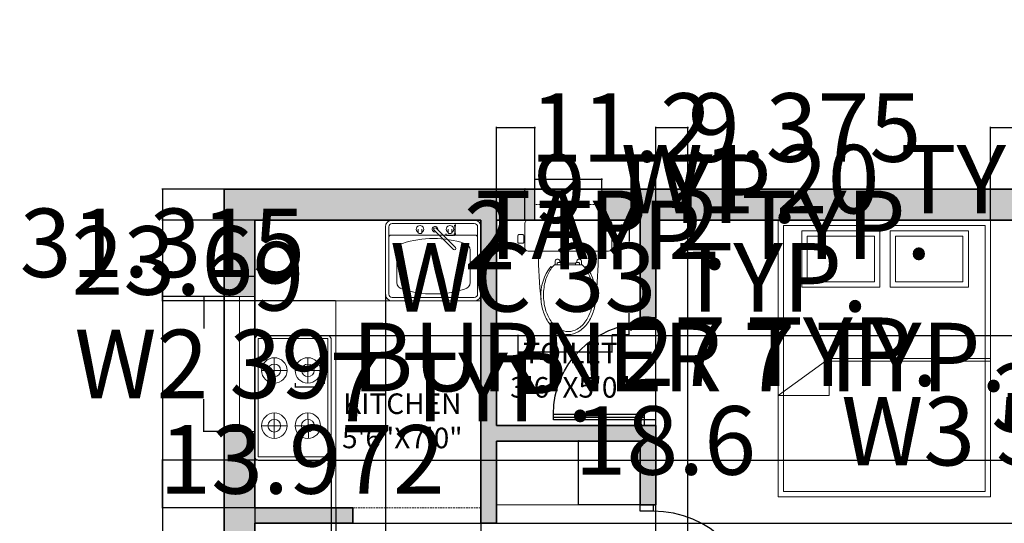
# Model space of a CAD drawing. Units: inches. Extents: x 305 to 776, y 38 to 479.
# Tile 13 of 14: x 331 to 618, y 332 to 479. Entities that reach past the tile are written whole.
import ezdxf

# ---------------------------------------------------------------- set-up
doc = ezdxf.new("R2010")
doc.units = ezdxf.units.IN
doc.header["$MEASUREMENT"] = 0
doc.linetypes.add('DASHED', pattern=[0.75, 0.5, -0.25])
for name, color, linetype, lineweight in [('A-ANNO-DIMS', 2, 'Continuous', 18), ('A-AREA-IDEN', 7, 'Continuous', 18), ('A-DOOR', 4, 'Continuous', 25), ('A-EQPM', 8, 'Continuous', 18), ('A-FLOR-CASE', 8, 'Continuous', 20), ('A-FLOR-FIXT', 9, 'Continuous', 18), ('A-FURN', 8, 'Continuous', 18), ('A-GLAZ', 4, 'Continuous', 20), ('A-GLAZ-OVHD', 4, 'DASHED', 18), ('A-WALL', 7, 'Continuous', 35), ('A-WALL-OVHD', 7, 'DASHED', 18), ('A-WALL-PATT', 252, 'Continuous', 13)]:
    doc.layers.add(name, color=color, linetype=linetype, lineweight=lineweight)
doc.styles.get("Standard").update_dxf_attribs({"font": 'arial.ttf'})
doc.dimstyles.get("Standard").update_dxf_attribs({"dimtxt": 20, "dimasz": 0.18, "dimexe": 0.18, "dimexo": 0.0625, "dimgap": 0.09, "dimtad": 0, "dimtih": 1, "dimtoh": 1, "dimdec": 4, "dimzin": 0, "dimdsep": 46, "dimtxsty": 'Standard', "dimcen": 0.09, "dimadec": 0, "dimazin": 0, "dimtfac": 1, "dimtdec": 4, "dimtofl": 0, "dimtmove": 0, "dimatfit": 3, "dimfxl": 1, "dimtolj": 1, "dimtzin": 0, "dimarcsym": 0})

# ---------------------------------------------------------------- blocks, each defined once
blk = doc.blocks.new('A$C296830DC')
blk.add_line((828.9, 852.6), (828.9, 94.7))
for points in [[(852.6, 94.7), (852.6, 852.6), (805.3, 852.6), (805.3, 94.7)], [(47.4, 94.7), (47.4, 0), (0, 0), (0, 94.7)], [(900, 94.7), (900, 0), (852.6, 0), (852.6, 94.7)]]:
    blk.add_lwpolyline(points, close=True)
blk.add_arc((805.3, 94.7), 757.9, 90, 180)
blk = doc.blocks.new('W1')
blk.add_line((867.01, 338.44), (847.41, 338.44))
blk.add_lwpolyline([(847.41, 333.94), (867.01, 333.94), (867.01, 342.94), (847.41, 342.94)], close=True)
blk = doc.blocks.new('t')
for points in [[(1220.28, 636.63), (1208.55, 636.63, 0.414214), (1207.58, 635.67), (1207.58, 631.86, 0.414214)], [(1220.28, 636.63), (1232.02, 636.63, -0.414214), (1232.98, 635.67), (1232.98, 628.51, -0.414214), (1232.02, 627.55), (1229.53, 627.55)], [(1207.31, 631.86), (1207.31, 632.04, 0.414214), (1206.99, 632.37), (1205.84, 632.37, 0.414214), (1205.52, 632.04), (1205.52, 630.21, 0.414214), (1205.84, 629.89)], [(1205.84, 629.89), (1206.99, 629.89, 0.414214), (1207.31, 630.21), (1207.31, 630.39, 0.414214)], [(1207.31, 630.39), (1207.31, 631.86, 0.414214)], [(1207.58, 631.86), (1207.58, 630.39, 0.414214)], [(1207.58, 630.39), (1207.58, 628.51, 0.414214), (1208.55, 627.55), (1211.03, 627.55)], [(1211.03, 627.55, -0.279901), (1211.54, 626.96, 0.030761), (1212.34, 613.45, 16.522544)], [(1229.53, 627.55, 0.279901), (1229.02, 626.96, -0.030761), (1228.22, 613.45, -16.522544)], [(1216.48, 623.56), (1216.48, 624.75, -0.788198), (1217.76, 624.75), (1217.76, 624.2)], [(1217.03, 623.56), (1217.03, 623.98, -0.414214), (1217.26, 624.2), (1217.94, 624.2, -0.414214), (1218.17, 623.98), (1218.17, 623.56)], [(1223.54, 623.56), (1223.54, 623.98, 0.414214), (1223.31, 624.2), (1222.62, 624.2, 0.414214), (1222.39, 623.98), (1222.39, 623.56)], [(1224.09, 623.56), (1224.09, 624.75, 0.788198), (1222.8, 624.75), (1222.8, 624.2)], [(1212.3, 614.03, -0.186192), (1215.17, 623.1), (1215.53, 622.81)], [(1213.04, 614.76, 0.068564), (1213.62, 610.52, 0.080689), (1215.16, 607.21, 0.107047), (1217.67, 604.81, 0.137952), (1220.28, 604.08, 0.137952), (1222.89, 604.81, 0.107047), (1225.4, 607.21, 0.080689), (1226.94, 610.52, 0.068564), (1227.53, 614.76, 0.068564), (1226.94, 619.01, 0.080689), (1225.4, 622.31, 0.049741), (1224.36, 623.56, 0.137952)], [(1216.2, 623.56, 0.049741), (1215.16, 622.31, 0.080689), (1213.62, 619.01, 0.068564), (1213.04, 614.76, 0.068564)], [(1228.22, 613.45, 0.197511), (1225.39, 623.1), (1225.04, 622.81)], [(1212.27, 614.03, 0.059006), (1212.9, 610.18, 0.081908), (1214.61, 606.59, 0.106902), (1217.38, 604.01, 0.135271), (1220.28, 603.21, 0.135271)], [(1212.34, 613.45, -0.010918), (1212.3, 614.03)], [(1220.28, 603.21, 0.135271), (1223.19, 604.01, 0.106902), (1225.95, 606.59, 0.081908), (1227.66, 610.18, 0.059006), (1228.29, 614.03, 0.070136)]]:
    blk.add_lwpolyline(points, format="xyb")
for points in [[(1207.31, 631.86), (1207.58, 631.86)], [(1207.31, 630.39), (1207.58, 630.39)], [(1211.03, 627.55), (1220.28, 627.55)], [(1229.53, 627.55), (1220.28, 627.55)], [(1218.17, 624.02), (1222.39, 624.02)], [(1216.2, 623.56), (1224.36, 623.56)]]:
    blk.add_lwpolyline(points)
blk = doc.blocks.new('BED')
for p, q in [((1579.44, 254.58), (1564.49, 243.77)), ((1564.49, 243.77), (1579.44, 254.58)), ((1626.49, 254.58), (1579.44, 254.58)), ((1579.44, 254.58), (1579.44, 243.77)), ((1626.49, 253.76), (1579.44, 253.76)), ((1579.44, 243.77), (1564.49, 243.77))]:
    blk.add_line(p, q)
for points in [[(1626.49, 214.2), (1564.49, 214.2), (1564.49, 294.96), (1626.49, 294.96)], [(1624.92, 215.77), (1566.06, 215.77), (1566.06, 293.39), (1624.92, 293.39)], [(1594.24, 275.39), (1571.42, 275.39), (1571.42, 291.78), (1594.24, 291.78)], [(1620.04, 275.39), (1597.22, 275.39), (1597.22, 291.78), (1620.04, 291.78)], [(1592.67, 276.96), (1572.99, 276.96), (1572.99, 290.21), (1592.67, 290.21)], [(1618.47, 276.96), (1598.79, 276.96), (1598.79, 290.21), (1618.47, 290.21)]]:
    blk.add_lwpolyline(points, close=True)
blk = doc.blocks.new('w2')
blk.add_line((795.76, 498.04), (795.76, 458.67))
blk.add_lwpolyline([(791.26, 458.67), (800.26, 458.67), (800.26, 498.04), (791.26, 498.04)], close=True)
blk = doc.blocks.new('COOKTOP-BURNER')
for p, q in [((3.71, 7.42), (3.71, 0)), ((7.42, 3.71), (0, 3.71))]:
    blk.add_line(p, q)
for radius in [3.71, 1.85]:
    blk.add_circle((3.71, 3.71), radius)
blk = doc.blocks.new('FAUCET-HANDLE')
for p, q in [((0.55, 0.18), (0.55, 1.27)), ((1.64, 0.18), (1.64, 1.27))]:
    blk.add_line(p, q)
for centre, radius, start, end in [((1.09, 1.27), 1.09, 300, 240), ((1.09, 0.93), 0.928, 233.9153, 306.0847)]:
    blk.add_arc(centre, radius, start, end)
blk = doc.blocks.new('*D23')
at = {"layer": 'A-ANNO-DIMS', "color": 0, "lineweight": -2, "transparency": 16777216}
for p, q in [((481.33, 429.44), (481.33, 432.5)), ((481.51, 432.32), (500.75, 432.32)), ((500.93, 429.44), (500.93, 432.5)), ((500.93, 432.32), (501.11, 432.32))]:
    blk.add_line(p, q, dxfattribs=at)
at = {"layer": 'A-ANNO-DIMS', "color": 0, "transparency": 16777216}
for points in [[(481.51, 432.35), (481.51, 432.29), (481.33, 432.32)], [(500.75, 432.35), (500.75, 432.29), (500.93, 432.32)]]:
    blk.add_solid(points, dxfattribs=at)
at = {"layer": 'Defpoints', "color": 0, "transparency": 16777216}
for p in [(500.93, 432.32), (481.33, 429.38), (500.93, 429.38)]:
    blk.add_point(p, dxfattribs=at)
at = {"layer": 'A-ANNO-DIMS', "color": 0, "transparency": 16777216, "insert": (575.13, 432.32), "char_height": 20, "attachment_point": 5}
blk.add_mtext('\\A1;W1 20 TYP.', dxfattribs=at)
blk = doc.blocks.new('*D24')
at = {"layer": 'A-ANNO-DIMS', "color": 0, "lineweight": -2, "transparency": 16777216}
for p, q in [((481.27, 429.38), (478.21, 429.38)), ((478.39, 429.38), (478.39, 429.56)), ((478.39, 429.56), (478.57, 429.56)), ((478.39, 420.56), (478.39, 429.2)), ((481.27, 420.38), (478.21, 420.38))]:
    blk.add_line(p, q, dxfattribs=at)
at = {"layer": 'A-ANNO-DIMS', "color": 0, "transparency": 16777216}
for points in [[(478.36, 429.2), (478.42, 429.2), (478.39, 429.38)], [(478.36, 420.56), (478.42, 420.56), (478.39, 420.38)]]:
    blk.add_solid(points, dxfattribs=at)
at = {"layer": 'Defpoints', "color": 0, "transparency": 16777216}
for p in [(478.39, 429.38), (481.33, 429.38), (481.33, 420.38)]:
    blk.add_point(p, dxfattribs=at)
at = {"layer": 'A-ANNO-DIMS', "color": 0, "transparency": 16777216, "insert": (519.57, 429.56), "char_height": 20, "attachment_point": 5}
blk.add_mtext('\\A1;9 TYP.', dxfattribs=at)
blk = doc.blocks.new('*D25')
at = {"layer": 'A-ANNO-DIMS', "color": 0, "lineweight": -2, "transparency": 16777216}
for p, q in [((390.57, 398.07), (384.55, 398.07)), ((384.73, 397.89), (384.73, 388.69)), ((384.73, 358.88), (384.73, 368.07)), ((390.57, 358.7), (384.55, 358.7))]:
    blk.add_line(p, q, dxfattribs=at)
at = {"layer": 'A-ANNO-DIMS', "color": 0, "transparency": 16777216}
for points in [[(384.7, 397.89), (384.76, 397.89), (384.73, 398.07)], [(384.7, 358.88), (384.76, 358.88), (384.73, 358.7)]]:
    blk.add_solid(points, dxfattribs=at)
at = {"layer": 'Defpoints', "color": 0, "transparency": 16777216}
for p in [(384.73, 398.07), (390.63, 398.07), (390.63, 358.7)]:
    blk.add_point(p, dxfattribs=at)
at = {"layer": 'A-ANNO-DIMS', "color": 0, "transparency": 16777216, "insert": (384.73, 378.38), "char_height": 20, "attachment_point": 5}
blk.add_mtext('\\A1;W2 39', dxfattribs=at)
blk = doc.blocks.new('*D26')
at = {"layer": 'A-ANNO-DIMS', "color": 0, "lineweight": -2, "transparency": 16777216}
for p, q in [((390.63, 398.13), (390.63, 404.15)), ((390.81, 403.97), (399.45, 403.97)), ((399.63, 398.13), (399.63, 404.15)), ((399.63, 403.97), (399.81, 403.97))]:
    blk.add_line(p, q, dxfattribs=at)
at = {"layer": 'A-ANNO-DIMS', "color": 0, "transparency": 16777216}
for points in [[(390.81, 404), (390.81, 403.94), (390.63, 403.97)], [(399.45, 404), (399.45, 403.94), (399.63, 403.97)]]:
    blk.add_solid(points, dxfattribs=at)
at = {"layer": 'Defpoints', "color": 0, "transparency": 16777216}
for p in [(399.63, 403.97), (390.63, 398.07), (399.63, 398.07)]:
    blk.add_point(p, dxfattribs=at)
at = {"layer": 'A-ANNO-DIMS', "color": 0, "transparency": 16777216, "insert": (406.48, 403.97), "char_height": 20, "attachment_point": 5}
blk.add_mtext('\\A1;9', dxfattribs=at)
blk = doc.blocks.new('*D27')
at = {"layer": 'A-ANNO-DIMS', "color": 0, "lineweight": -2, "transparency": 16777216}
for p, q in [((630.7, 388.18), (639.63, 388.18)), ((639.45, 388), (639.45, 369.09)), ((639.45, 329.56), (639.45, 348.47)), ((630.7, 329.38), (639.63, 329.38))]:
    blk.add_line(p, q, dxfattribs=at)
at = {"layer": 'A-ANNO-DIMS', "color": 0, "transparency": 16777216}
for points in [[(639.42, 388), (639.48, 388), (639.45, 388.18)], [(639.42, 329.56), (639.48, 329.56), (639.45, 329.38)]]:
    blk.add_solid(points, dxfattribs=at)
at = {"layer": 'Defpoints', "color": 0, "transparency": 16777216}
for p in [(630.63, 388.18), (630.63, 329.38), (639.45, 329.38)]:
    blk.add_point(p, dxfattribs=at)
at = {"layer": 'A-ANNO-DIMS', "color": 0, "transparency": 16777216, "insert": (639.45, 358.78), "char_height": 20, "attachment_point": 5}
blk.add_mtext('\\A1;W3 59 TYP.', dxfattribs=at)
blk = doc.blocks.new('*D31')
at = {"layer": 'A-ANNO-DIMS', "color": 0, "lineweight": -2, "transparency": 16777216}
for p, q in [((503.89, 420.38), (509.03, 420.38)), ((508.85, 420.2), (508.85, 414.11)), ((508.85, 387.14), (508.85, 393.23)), ((503.89, 386.96), (509.03, 386.96))]:
    blk.add_line(p, q, dxfattribs=at)
at = {"layer": 'A-ANNO-DIMS', "color": 0, "transparency": 16777216}
for points in [[(508.82, 420.2), (508.88, 420.2), (508.85, 420.38)], [(508.82, 387.14), (508.88, 387.14), (508.85, 386.96)]]:
    blk.add_solid(points, dxfattribs=at)
at = {"layer": 'Defpoints', "color": 0, "transparency": 16777216}
for p in [(503.83, 420.38), (508.85, 420.38), (503.83, 386.96)]:
    blk.add_point(p, dxfattribs=at)
at = {"layer": 'A-ANNO-DIMS', "color": 0, "transparency": 16777216, "insert": (508.85, 403.67), "char_height": 20, "attachment_point": 5}
blk.add_mtext('\\A1;WC 33 TYP.', dxfattribs=at)
blk = doc.blocks.new('*D32')
at = {"layer": 'A-ANNO-DIMS', "color": 0, "lineweight": -2, "transparency": 16777216}
for p, q in [((476.37, 386.9), (476.37, 381.77)), ((503.83, 386.9), (503.83, 381.77)), ((476.55, 381.95), (503.65, 381.95)), ((503.83, 381.95), (504.01, 381.95))]:
    blk.add_line(p, q, dxfattribs=at)
at = {"layer": 'A-ANNO-DIMS', "color": 0, "transparency": 16777216}
for points in [[(476.55, 381.98), (476.55, 381.92), (476.37, 381.95)], [(503.65, 381.98), (503.65, 381.92), (503.83, 381.95)]]:
    blk.add_solid(points, dxfattribs=at)
at = {"layer": 'Defpoints', "color": 0, "transparency": 16777216}
for p in [(476.37, 386.96), (503.83, 386.96), (503.83, 381.95)]:
    blk.add_point(p, dxfattribs=at)
at = {"layer": 'A-ANNO-DIMS', "color": 0, "transparency": 16777216, "insert": (552.95, 381.95), "char_height": 20, "attachment_point": 5}
blk.add_mtext('\\A1;27 TYP.', dxfattribs=at)
blk = doc.blocks.new('*D41')
at = {"layer": 'A-ANNO-DIMS', "color": 0, "lineweight": -2, "transparency": 16777216}
for p, q in [((418.87, 380.22), (420.1, 380.22)), ((419.92, 380.22), (419.92, 380.4)), ((419.92, 380.4), (420.1, 380.4)), ((419.92, 372.98), (419.92, 380.04)), ((418.87, 372.8), (420.1, 372.8))]:
    blk.add_line(p, q, dxfattribs=at)
at = {"layer": 'A-ANNO-DIMS', "color": 0, "transparency": 16777216}
for points in [[(419.89, 380.04), (419.95, 380.04), (419.92, 380.22)], [(419.89, 372.98), (419.95, 372.98), (419.92, 372.8)]]:
    blk.add_solid(points, dxfattribs=at)
at = {"layer": 'Defpoints', "color": 0, "transparency": 16777216}
for p in [(418.81, 380.22), (419.92, 380.22), (418.81, 372.8)]:
    blk.add_point(p, dxfattribs=at)
at = {"layer": 'A-ANNO-DIMS', "color": 0, "transparency": 16777216, "insert": (523.52, 380.4), "char_height": 20, "attachment_point": 5}
blk.add_mtext('\\A1;BURNER 7 TYP.', dxfattribs=at)
blk = doc.blocks.new('*D42')
at = {"layer": 'A-ANNO-DIMS', "color": 0, "lineweight": -2, "transparency": 16777216}
for p, q in [((411.39, 372.73), (411.39, 371.5)), ((411.57, 371.68), (418.63, 371.68)), ((418.81, 372.73), (418.81, 371.5)), ((418.81, 371.68), (418.99, 371.68))]:
    blk.add_line(p, q, dxfattribs=at)
at = {"layer": 'A-ANNO-DIMS', "color": 0, "transparency": 16777216}
for points in [[(411.57, 371.71), (411.57, 371.65), (411.39, 371.68)], [(418.63, 371.71), (418.63, 371.65), (418.81, 371.68)]]:
    blk.add_solid(points, dxfattribs=at)
at = {"layer": 'Defpoints', "color": 0, "transparency": 16777216}
for p in [(411.39, 372.8), (418.81, 372.8), (418.81, 371.68)]:
    blk.add_point(p, dxfattribs=at)
at = {"layer": 'A-ANNO-DIMS', "color": 0, "transparency": 16777216, "insert": (459.9, 371.68), "char_height": 20, "attachment_point": 5}
blk.add_mtext('\\A1;7 TYP.', dxfattribs=at)
blk = doc.blocks.new('*D43')
at = {"layer": 'A-ANNO-DIMS', "color": 0, "lineweight": -2, "transparency": 16777216}
for p, q in [((457.83, 418.8), (458.31, 418.8)), ((458.13, 418.8), (458.13, 418.98)), ((458.13, 418.98), (458.31, 418.98)), ((458.13, 416.56), (458.13, 418.62)), ((457.83, 416.38), (458.31, 416.38))]:
    blk.add_line(p, q, dxfattribs=at)
at = {"layer": 'A-ANNO-DIMS', "color": 0, "transparency": 16777216}
for points in [[(458.1, 418.62), (458.16, 418.62), (458.13, 418.8)], [(458.1, 416.56), (458.16, 416.56), (458.13, 416.38)]]:
    blk.add_solid(points, dxfattribs=at)
at = {"layer": 'Defpoints', "color": 0, "transparency": 16777216}
for p in [(457.77, 418.8), (458.13, 418.8), (457.77, 416.38)]:
    blk.add_point(p, dxfattribs=at)
at = {"layer": 'A-ANNO-DIMS', "color": 0, "transparency": 16777216, "insert": (530.61, 418.98), "char_height": 20, "attachment_point": 5}
blk.add_mtext('\\A1;TAP 2 TYP.', dxfattribs=at)
blk = doc.blocks.new('*D44')
at = {"layer": 'A-ANNO-DIMS', "color": 0, "lineweight": -2, "transparency": 16777216}
for p, q in [((455.4, 416.31), (455.4, 415.83)), ((455.58, 416.01), (457.59, 416.01)), ((457.77, 416.31), (457.77, 415.83)), ((457.77, 416.01), (457.95, 416.01))]:
    blk.add_line(p, q, dxfattribs=at)
at = {"layer": 'A-ANNO-DIMS', "color": 0, "transparency": 16777216}
for points in [[(455.58, 416.04), (455.58, 415.98), (455.4, 416.01)], [(457.59, 416.04), (457.59, 415.98), (457.77, 416.01)]]:
    blk.add_solid(points, dxfattribs=at)
at = {"layer": 'Defpoints', "color": 0, "transparency": 16777216}
for p in [(455.4, 416.38), (457.77, 416.38), (457.77, 416.01)]:
    blk.add_point(p, dxfattribs=at)
at = {"layer": 'A-ANNO-DIMS', "color": 0, "transparency": 16777216, "insert": (499.12, 416.01), "char_height": 20, "attachment_point": 5}
blk.add_mtext('\\A1;2 TYP.', dxfattribs=at)
blk = doc.blocks.new('*D46')
at = {"layer": 'A-ANNO-DIMS', "color": 0, "lineweight": -2, "transparency": 16777216}
for p, q in [((390.57, 429.38), (372.45, 429.38)), ((372.63, 429.2), (372.63, 259.69)), ((372.63, 69.56), (372.63, 239.07)), ((390.57, 69.38), (372.45, 69.38))]:
    blk.add_line(p, q, dxfattribs=at)
at = {"layer": 'A-ANNO-DIMS', "color": 0, "transparency": 16777216}
for points in [[(372.6, 429.2), (372.66, 429.2), (372.63, 429.38)], [(372.6, 69.56), (372.66, 69.56), (372.63, 69.38)]]:
    blk.add_solid(points, dxfattribs=at)
at = {"layer": 'Defpoints', "color": 0, "transparency": 16777216}
for p in [(372.63, 429.38), (390.63, 429.38), (390.63, 69.38)]:
    blk.add_point(p, dxfattribs=at)
at = {"layer": 'A-ANNO-DIMS', "color": 0, "transparency": 16777216, "insert": (372.63, 249.38), "char_height": 20, "attachment_point": 5}
blk.add_mtext('\\A1;360', dxfattribs=at)
blk = doc.blocks.new('*D49')
at = {"layer": 'A-ANNO-DIMS', "color": 0, "lineweight": -2, "transparency": 16777216}
for p, q in [((399.7, 331.88), (648.81, 331.88)), ((648.63, 331.7), (648.63, 330.88)), ((399.7, 309.28), (648.81, 309.28)), ((648.63, 309.46), (648.63, 310.28))]:
    blk.add_line(p, q, dxfattribs=at)
at = {"layer": 'A-ANNO-DIMS', "color": 0, "transparency": 16777216}
for points in [[(648.6, 331.7), (648.66, 331.7), (648.63, 331.88)], [(648.6, 309.46), (648.66, 309.46), (648.63, 309.28)]]:
    blk.add_solid(points, dxfattribs=at)
at = {"layer": 'Defpoints', "color": 0, "transparency": 16777216}
for p in [(399.63, 331.88), (648.63, 331.88), (399.63, 309.28)]:
    blk.add_point(p, dxfattribs=at)
at = {"layer": 'A-ANNO-DIMS', "color": 0, "transparency": 16777216, "insert": (648.63, 320.58), "char_height": 20, "attachment_point": 5}
blk.add_mtext('\\A1;22.6', dxfattribs=at)
blk = doc.blocks.new('*D50')
at = {"layer": 'A-ANNO-DIMS', "color": 0, "lineweight": -2, "transparency": 16777216}
for p, q in [((390.57, 429.38), (372.45, 429.38)), ((372.63, 429.2), (372.63, 424.03)), ((372.63, 398.25), (372.63, 403.42)), ((390.57, 398.07), (372.45, 398.07))]:
    blk.add_line(p, q, dxfattribs=at)
at = {"layer": 'A-ANNO-DIMS', "color": 0, "transparency": 16777216}
for points in [[(372.6, 429.2), (372.66, 429.2), (372.63, 429.38)], [(372.6, 398.25), (372.66, 398.25), (372.63, 398.07)]]:
    blk.add_solid(points, dxfattribs=at)
at = {"layer": 'Defpoints', "color": 0, "transparency": 16777216}
for p in [(390.63, 429.38), (372.63, 398.07), (390.63, 398.07)]:
    blk.add_point(p, dxfattribs=at)
at = {"layer": 'A-ANNO-DIMS', "color": 0, "transparency": 16777216, "insert": (372.63, 413.72), "char_height": 20, "attachment_point": 5}
blk.add_mtext('\\A1;31.315', dxfattribs=at)
blk = doc.blocks.new('*D54')
at = {"layer": 'A-ANNO-DIMS', "color": 0, "lineweight": -2, "transparency": 16777216}
for p, q in [((470.13, 420.44), (470.13, 447.56)), ((470.31, 447.38), (481.15, 447.38)), ((481.33, 420.44), (481.33, 447.56)), ((481.33, 447.38), (481.51, 447.38))]:
    blk.add_line(p, q, dxfattribs=at)
at = {"layer": 'A-ANNO-DIMS', "color": 0, "transparency": 16777216}
for points in [[(470.31, 447.41), (470.31, 447.35), (470.13, 447.38)], [(481.15, 447.41), (481.15, 447.35), (481.33, 447.38)]]:
    blk.add_solid(points, dxfattribs=at)
at = {"layer": 'Defpoints', "color": 0, "transparency": 16777216}
for p in [(481.33, 447.38), (470.13, 420.38), (481.33, 420.38)]:
    blk.add_point(p, dxfattribs=at)
at = {"layer": 'A-ANNO-DIMS', "color": 0, "transparency": 16777216, "insert": (506.53, 447.38), "char_height": 20, "attachment_point": 5}
blk.add_mtext('\\A1;11.2', dxfattribs=at)
blk = doc.blocks.new('*D58')
at = {"layer": 'A-ANNO-DIMS', "color": 0, "lineweight": -2, "transparency": 16777216}
for p, q in [((516.63, 138.44), (516.63, 447.56)), ((516.81, 447.38), (525.83, 447.38)), ((526.01, 138.44), (526.01, 447.56)), ((526.01, 447.38), (526.19, 447.38))]:
    blk.add_line(p, q, dxfattribs=at)
at = {"layer": 'A-ANNO-DIMS', "color": 0, "transparency": 16777216}
for points in [[(516.81, 447.41), (516.81, 447.35), (516.63, 447.38)], [(525.83, 447.41), (525.83, 447.35), (526.01, 447.38)]]:
    blk.add_solid(points, dxfattribs=at)
at = {"layer": 'Defpoints', "color": 0, "transparency": 16777216}
for p in [(526.01, 447.38), (516.63, 138.38), (526.01, 138.38)]:
    blk.add_point(p, dxfattribs=at)
at = {"layer": 'A-ANNO-DIMS', "color": 0, "transparency": 16777216, "insert": (560.1, 447.38), "char_height": 20, "attachment_point": 5}
blk.add_mtext('\\A1;9.375', dxfattribs=at)
blk = doc.blocks.new('*D61')
at = {"layer": 'A-ANNO-DIMS', "color": 0, "lineweight": -2, "transparency": 16777216}
for p, q in [((437.73, 398.69), (437.73, 51.2)), ((465.63, 398.69), (465.63, 51.2)), ((437.91, 51.38), (465.45, 51.38)), ((465.63, 51.38), (465.81, 51.38))]:
    blk.add_line(p, q, dxfattribs=at)
at = {"layer": 'A-ANNO-DIMS', "color": 0, "transparency": 16777216}
for points in [[(437.91, 51.41), (437.91, 51.35), (437.73, 51.38)], [(465.45, 51.41), (465.45, 51.35), (465.63, 51.38)]]:
    blk.add_solid(points, dxfattribs=at)
at = {"layer": 'Defpoints', "color": 0, "transparency": 16777216}
for p in [(437.73, 398.75), (465.63, 398.75), (465.63, 51.38)]:
    blk.add_point(p, dxfattribs=at)
at = {"layer": 'A-ANNO-DIMS', "color": 0, "transparency": 16777216, "insert": (492.07, 51.38), "char_height": 20, "attachment_point": 5}
blk.add_mtext('\\A1;27.9', dxfattribs=at)
blk = doc.blocks.new('*D62')
at = {"layer": 'A-ANNO-DIMS', "color": 0, "lineweight": -2, "transparency": 16777216}
for p, q in [((399.63, 336.32), (399.63, 51.2)), ((423.23, 336.32), (423.23, 51.2)), ((399.81, 51.38), (423.05, 51.38)), ((423.23, 51.38), (423.41, 51.38))]:
    blk.add_line(p, q, dxfattribs=at)
at = {"layer": 'A-ANNO-DIMS', "color": 0, "transparency": 16777216}
for points in [[(399.81, 51.41), (399.81, 51.35), (399.63, 51.38)], [(423.05, 51.41), (423.05, 51.35), (423.23, 51.38)]]:
    blk.add_solid(points, dxfattribs=at)
at = {"layer": 'Defpoints', "color": 0, "transparency": 16777216}
for p in [(399.63, 336.38), (423.23, 336.38), (423.23, 51.38)]:
    blk.add_point(p, dxfattribs=at)
at = {"layer": 'A-ANNO-DIMS', "color": 0, "transparency": 16777216, "insert": (449.64, 51.38), "char_height": 20, "attachment_point": 5}
blk.add_mtext('\\A1;23.6', dxfattribs=at)
blk = doc.blocks.new('*D63')
at = {"layer": 'A-ANNO-DIMS', "color": 0, "lineweight": -2, "transparency": 16777216}
for p, q in [((399.57, 420.38), (372.45, 420.38)), ((372.63, 420.2), (372.63, 418.89)), ((423.17, 396.78), (372.45, 396.78)), ((372.63, 396.96), (372.63, 398.27))]:
    blk.add_line(p, q, dxfattribs=at)
at = {"layer": 'A-ANNO-DIMS', "color": 0, "transparency": 16777216}
for points in [[(372.6, 420.2), (372.66, 420.2), (372.63, 420.38)], [(372.6, 396.96), (372.66, 396.96), (372.63, 396.78)]]:
    blk.add_solid(points, dxfattribs=at)
at = {"layer": 'Defpoints', "color": 0, "transparency": 16777216}
for p in [(372.63, 420.38), (399.63, 420.38), (423.23, 396.78)]:
    blk.add_point(p, dxfattribs=at)
at = {"layer": 'A-ANNO-DIMS', "color": 0, "transparency": 16777216, "insert": (372.63, 408.58), "char_height": 20, "attachment_point": 5}
blk.add_mtext('\\A1;23.6', dxfattribs=at)
blk = doc.blocks.new('*D64')
at = {"layer": 'A-ANNO-DIMS', "color": 0, "lineweight": -2, "transparency": 16777216}
for p, q in [((400.62, 386.71), (648.81, 386.71)), ((648.63, 386.53), (648.63, 378.84)), ((648.63, 350.53), (648.63, 358.22)), ((400.62, 350.35), (648.81, 350.35))]:
    blk.add_line(p, q, dxfattribs=at)
at = {"layer": 'A-ANNO-DIMS', "color": 0, "transparency": 16777216}
for points in [[(648.6, 386.53), (648.66, 386.53), (648.63, 386.71)], [(648.6, 350.53), (648.66, 350.53), (648.63, 350.35)]]:
    blk.add_solid(points, dxfattribs=at)
at = {"layer": 'Defpoints', "color": 0, "transparency": 16777216}
for p in [(400.56, 386.71), (648.63, 386.71), (400.56, 350.35)]:
    blk.add_point(p, dxfattribs=at)
at = {"layer": 'A-ANNO-DIMS', "color": 0, "transparency": 16777216, "insert": (648.63, 368.53), "char_height": 20, "attachment_point": 5}
blk.add_mtext('\\A1;36.35', dxfattribs=at)
blk = doc.blocks.new('*D65')
at = {"layer": 'A-ANNO-DIMS', "color": 0, "lineweight": -2, "transparency": 16777216}
for p, q in [((399.63, 351.22), (399.63, 51.2)), ((421.89, 351.22), (421.89, 51.2)), ((399.81, 51.38), (421.71, 51.38)), ((421.89, 51.38), (422.07, 51.38))]:
    blk.add_line(p, q, dxfattribs=at)
at = {"layer": 'A-ANNO-DIMS', "color": 0, "transparency": 16777216}
for points in [[(399.81, 51.41), (399.81, 51.35), (399.63, 51.38)], [(421.71, 51.41), (421.71, 51.35), (421.89, 51.38)]]:
    blk.add_solid(points, dxfattribs=at)
at = {"layer": 'Defpoints', "color": 0, "transparency": 16777216}
for p in [(399.63, 351.28), (421.89, 351.28), (421.89, 51.38)]:
    blk.add_point(p, dxfattribs=at)
at = {"layer": 'A-ANNO-DIMS', "color": 0, "transparency": 16777216, "insert": (463.84, 51.38), "char_height": 20, "attachment_point": 5}
blk.add_mtext('\\A1;22.257', dxfattribs=at)
blk = doc.blocks.new('*D66')
at = {"layer": 'A-ANNO-DIMS', "color": 0, "lineweight": -2, "transparency": 16777216}
for p, q in [((400.5, 350.35), (372.45, 350.35)), ((372.63, 350.35), (372.63, 350.53)), ((372.63, 350.53), (372.81, 350.53)), ((372.63, 336.56), (372.63, 350.17)), ((423.17, 336.38), (372.45, 336.38))]:
    blk.add_line(p, q, dxfattribs=at)
at = {"layer": 'A-ANNO-DIMS', "color": 0, "transparency": 16777216}
for points in [[(372.6, 350.17), (372.66, 350.17), (372.63, 350.35)], [(372.6, 336.56), (372.66, 336.56), (372.63, 336.38)]]:
    blk.add_solid(points, dxfattribs=at)
at = {"layer": 'Defpoints', "color": 0, "transparency": 16777216}
for p in [(372.63, 350.35), (400.56, 350.35), (423.23, 336.38)]:
    blk.add_point(p, dxfattribs=at)
at = {"layer": 'A-ANNO-DIMS', "color": 0, "transparency": 16777216, "insert": (413.37, 350.53), "char_height": 20, "attachment_point": 5}
blk.add_mtext('\\A1;13.972', dxfattribs=at)
blk = doc.blocks.new('*D68')
at = {"layer": 'A-ANNO-DIMS', "color": 0, "lineweight": -2, "transparency": 16777216}
for p, q in [((614.36, 420.44), (614.36, 447.56)), ((614.54, 447.38), (621.45, 447.38)), ((621.63, 420.44), (621.63, 447.56)), ((621.63, 447.38), (621.81, 447.38))]:
    blk.add_line(p, q, dxfattribs=at)
at = {"layer": 'A-ANNO-DIMS', "color": 0, "transparency": 16777216}
for points in [[(614.54, 447.41), (614.54, 447.35), (614.36, 447.38)], [(621.45, 447.41), (621.45, 447.35), (621.63, 447.38)]]:
    blk.add_solid(points, dxfattribs=at)
at = {"layer": 'Defpoints', "color": 0, "transparency": 16777216}
for p in [(621.63, 447.38), (614.36, 420.38), (621.63, 420.38)]:
    blk.add_point(p, dxfattribs=at)
at = {"layer": 'A-ANNO-DIMS', "color": 0, "transparency": 16777216, "insert": (653.64, 447.38), "char_height": 20, "attachment_point": 5}
blk.add_mtext('\\A1;7.271', dxfattribs=at)
blk = doc.blocks.new('*D71')
at = {"layer": 'A-ANNO-DIMS', "color": 0, "lineweight": -2, "transparency": 16777216}
for p, q in [((512.07, 355.88), (493.95, 355.88)), ((494.13, 355.88), (494.13, 356.06)), ((494.13, 356.06), (494.31, 356.06)), ((494.13, 337.46), (494.13, 355.7)), ((512.07, 337.28), (493.95, 337.28))]:
    blk.add_line(p, q, dxfattribs=at)
at = {"layer": 'A-ANNO-DIMS', "color": 0, "transparency": 16777216}
for points in [[(494.1, 355.7), (494.16, 355.7), (494.13, 355.88)], [(494.1, 337.46), (494.16, 337.46), (494.13, 337.28)]]:
    blk.add_solid(points, dxfattribs=at)
at = {"layer": 'Defpoints', "color": 0, "transparency": 16777216}
for p in [(494.13, 355.88), (512.13, 355.88), (512.13, 337.28)]:
    blk.add_point(p, dxfattribs=at)
at = {"layer": 'A-ANNO-DIMS', "color": 0, "transparency": 16777216, "insert": (519.43, 356.06), "char_height": 20, "attachment_point": 5}
blk.add_mtext('\\A1;18.6', dxfattribs=at)

msp = doc.modelspace()

# ---------------------------------------------------------------- hatches: boundary and pattern name
at = {"layer": 'A-WALL-PATT'}
h = msp.add_hatch(color=256, dxfattribs=at)
h.dxf.hatch_style = 1
h.paths.add_polyline_path([(481.3329, 429.382), (390.6329, 429.382), (390.6329, 398.067), (399.6329, 398.067), (399.6329, 420.382), (465.6329, 420.382), (465.6329, 331.882), (470.1329, 331.882), (470.1329, 355.882), (512.1329, 355.882), (512.1329, 337.282), (512.1329, 337.282), (515.8592, 337.282), (516.6329, 337.282), (516.6329, 360.382), (513.3171, 360.382), (470.1329, 360.382), (470.1329, 420.382), (481.3329, 420.382)])
h.paths.add_polyline_path([(630.6329, 429.382), (500.9329, 429.382), (500.9329, 420.382), (502.8693, 420.382), (512.1329, 420.382), (512.1329, 391.882), (516.6329, 391.882), (516.6329, 420.382), (621.6329, 420.382), (621.6329, 388.182), (630.6329, 388.182)])
h.paths.add_polyline_path([(630.6329, 329.382), (621.6329, 329.382), (621.6329, 301.882), (512.1329, 301.882), (512.1329, 297.382), (515.8592, 297.382), (557.6329, 297.382), (621.6329, 297.382), (621.6329, 286.182), (630.6329, 286.182)])
h.paths.add_polyline_path([(630.6329, 266.582), (621.6329, 266.582), (621.6329, 255.382), (589.1329, 255.382), (589.1329, 250.882), (621.6329, 250.882), (621.6329, 226.282), (630.6329, 226.282)])
h.paths.add_polyline_path([(630.6329, 167.482), (621.6329, 167.482), (621.6329, 149.1444), (621.6329, 142.882), (516.6329, 142.882), (516.6329, 261.982), (512.1329, 261.982), (512.1329, 138.382), (621.6329, 138.382), (621.6329, 78.382), (512.1329, 78.382), (512.1329, 69.382), (630.6329, 69.382)])
h.paths.add_polyline_path([(464.1329, 138.382), (476.7329, 138.382), (476.7329, 142.1084), (476.7329, 142.882), (459.6329, 142.882), (459.6329, 78.382), (399.6329, 78.382), (399.6329, 98.582), (390.6329, 98.582), (390.6329, 69.382), (464.1329, 69.382)])
h.paths.add_polyline_path([(459.6329, 142.882), (439.3329, 142.882), (439.3329, 138.382), (459.6329, 138.382)], flags=17)
h.paths.add_polyline_path([(399.6329, 138.382), (403.9329, 138.382), (403.9329, 141.5545), (403.9329, 141.5545), (403.9329, 142.882), (399.6329, 142.882), (399.6329, 250.4819), (390.6329, 250.4819), (390.6329, 118.182), (399.6329, 118.182)])
h.paths.add_polyline_path([(399.6329, 331.882), (428.2629, 331.882), (428.2629, 336.382), (399.6329, 336.382), (399.6329, 358.697), (390.6329, 358.697), (390.6329, 309.2819), (399.6329, 309.2819)])

# ---------------------------------------------------------------- linework, layer by layer
at = {"layer": 'A-EQPM'}
for p, q in [((399.6329, 386.7066), (399.6329, 350.3541)), ((400.5603, 386.7066), (420.9622, 386.7066)), ((400.5603, 385.7793), (400.5603, 351.2815)), ((400.5603, 385.7793), (420.9622, 385.7793)), ((420.9622, 386.7066), (420.9622, 386.7016)), ((420.9622, 385.7793), (420.9622, 351.2815)), ((421.8895, 385.7834), (421.8895, 351.2815)), ((415.0965, 364.0791), (415.2527, 356.6635)), ((405.3095, 360.3696), (409.0189, 360.3696)), ((418.806, 360.3696), (411.3871, 360.3696)), ((400.5603, 351.2815), (420.9622, 351.2815)), ((400.3441, 350.3541), (420.9622, 350.3541))]:
    msp.add_line(p, q, dxfattribs=at)
for radius in [3.7094, 1.8547]:
    msp.add_circle((415.0965, 360.3696), radius, dxfattribs=at)
for centre, radius, start, end in [((400.9641, 385.3755), 1.391, 106.874566, 163.125441), ((420.4738, 385.2809), 1.5022, 19.539718, 72.137641), ((400.4522, 351.1734), 0.8264, 172.484866, 277.515134), ((420.5584, 351.6853), 1.391, 286.874555, 343.125445)]:
    msp.add_arc(centre, radius, start, end, dxfattribs=at)
at = {"layer": 'A-FLOR-CASE'}
for p, q in [((465.6329, 396.782), (423.2329, 396.782)), ((423.2329, 396.782), (423.2329, 336.382)), ((512.1329, 337.282), (470.1329, 337.282))]:
    msp.add_line(p, q, dxfattribs=at)
at = {"layer": 'A-FLOR-FIXT'}
for p, q in [((463.6662, 420.382), (439.697, 420.382)), ((437.7303, 418.4154), (437.7303, 398.7487)), ((439.697, 419.3987), (463.6662, 419.3987)), ((451.9261, 417.4155), (457.5756, 411.766)), ((458.155, 412.3454), (452.5056, 417.9949)), ((465.6329, 398.7487), (465.6329, 418.4154)), ((463.9297, 416.0117), (439.3692, 416.0117)), ((441.6343, 416.0117), (439.3692, 416.0117)), ((441.0665, 411.5867), (441.0665, 402.1904)), ((462.4813, 402.1904), (462.4813, 411.5867)), ((439.697, 397.7654), (463.6662, 397.7654)), ((463.6662, 396.782), (439.697, 396.782))]:
    msp.add_line(p, q, dxfattribs=at)
for points in [[(438.7136, 418.4154), (438.7136, 398.7487)], [(464.6496, 398.7487), (464.6496, 418.4154)]]:
    msp.add_lwpolyline(points, dxfattribs=at)
for points in [[(442.7276, 413.5748, -0.15464107), (460.8202, 413.5748)], [(442.7276, 400.2023, 0.15464107), (460.8202, 400.2023, -0.02214818)]]:
    msp.add_lwpolyline(points, format="xyb", dxfattribs=at)
for centre, radius, start, end in [((439.697, 418.4154), 1.9667, 90, 180), ((463.6662, 418.4154), 1.9667, 0, 90), ((439.697, 418.4154), 0.9833, 90, 180), ((452.2158, 417.7052), 0.8194, 345, 285), ((452.2158, 417.7052), 0.4097, 45, 225), ((463.6662, 418.4154), 0.9833, 0, 90), ((439.3692, 415.3561), 0.6556, 90, 180), ((463.994, 415.3561), 0.6556, 0, 90), ((443.1051, 411.5713), 2.0387, 100.670755, 179.56936), ((457.8653, 412.0557), 0.4097, 225, 45), ((460.4427, 411.5713), 2.0387, 0.43064, 79.329245), ((443.1051, 402.2057), 2.0387, 180.43064, 259.329245), ((460.4427, 402.2057), 2.0387, 280.670755, 359.56936), ((439.697, 398.7487), 1.9667, 180, 270), ((439.697, 398.7487), 0.9833, 180, 270), ((463.6662, 398.7487), 1.9667, 270, 0), ((463.6662, 398.7487), 0.9833, 270, 0)]:
    msp.add_arc(centre, radius, start, end, dxfattribs=at)
at = {"layer": 'A-WALL'}
for p, q in [((399.6329, 420.382), (399.6329, 336.382)), ((465.6329, 420.382), (399.6329, 420.382)), ((465.6329, 420.382), (465.6329, 331.882)), ((470.1329, 420.382), (470.1329, 360.382)), ((512.1329, 420.382), (470.1329, 420.382)), ((512.1329, 420.382), (512.1329, 391.882)), ((621.6329, 420.382), (516.6329, 420.382)), ((516.6329, 420.382), (516.6329, 391.882)), ((516.6329, 391.882), (512.1329, 391.882)), ((516.6329, 360.382), (470.1329, 360.382)), ((516.6329, 360.382), (516.6329, 337.282)), ((512.1329, 355.882), (470.1329, 355.882)), ((470.1329, 355.882), (470.1329, 331.882)), ((512.1329, 355.882), (512.1329, 337.282)), ((428.2629, 336.382), (399.6329, 336.382)), ((428.2629, 336.382), (428.2629, 331.882)), ((516.6329, 337.282), (512.1329, 337.282)), ((399.6329, 331.882), (399.6329, 142.882)), ((428.2629, 331.882), (399.6329, 331.882)), ((470.1329, 331.882), (465.6329, 331.882))]:
    msp.add_line(p, q, dxfattribs=at)
msp.add_lwpolyline([(390.6329, 69.382), (630.6329, 69.382), (630.6329, 429.382), (390.6329, 429.382)], close=True, dxfattribs=at)
at = {"layer": 'A-WALL-OVHD'}
for p, q in [((428.2629, 336.382), (465.6329, 336.382)), ((465.6329, 331.882), (428.2629, 331.882))]:
    msp.add_line(p, q, dxfattribs=at)

# ---------------------------------------------------------------- block references
at = {"layer": 'A-DOOR'}
for p, xscale, yscale, zscale, rotation in [((516.6329, 391.882), -0.035, 0.035, 0.035, 90), ((512.1329, 337.282), 0.0393333333333333, 0.0393333333333333, 0.0393333333333333, 270)]:
    msp.add_blockref('A$C296830DC', p, dxfattribs=dict(at, xscale=xscale, yscale=yscale, zscale=zscale, rotation=rotation))
at = {"layer": 'A-EQPM'}
for p, rotation in [((409.0189, 372.7962), 90.00000000000088), ((401.6, 364.0791), 270.0000000000009)]:
    msp.add_blockref('COOKTOP-BURNER', p, dxfattribs=dict(at, rotation=rotation))
msp.add_blockref('COOKTOP-BURNER', (411.3871, 372.7962), dxfattribs=at)
at = {"layer": 'A-FLOR-FIXT'}
for name, p in [('t', (-729.1486, -216.2468)), ('FAUCET-HANDLE', (446.7528, 416.4346)), ('FAUCET-HANDLE', (455.4935, 416.4346))]:
    msp.add_blockref(name, p, dxfattribs=at)
at = {"layer": 'A-FURN'}
msp.add_blockref('BED', (-1012.1314, 125.4231), dxfattribs=at)
at = {"layer": 'A-GLAZ'}
msp.add_blockref('w2', (-400.6245, -99.9693), dxfattribs=at)
at = {"layer": 'A-GLAZ-OVHD'}
msp.add_blockref('W1', (-366.0792, 86.4392), dxfattribs=at)

# ---------------------------------------------------------------- texts
at = {"layer": 'A-AREA-IDEN', "char_height": 6, "attachment_point": 1}
for s, insert in [('\\pxqc;TOILET\\P3\'6"X5\'0"', (452.6598, 384.5554)), ('\\pxqc;KITCHEN\\P5\'6"X7\'0"', (403.5717, 369.7851))]:
    msp.add_mtext_dynamic_manual_height_columns(s, width=78.185, gutter_width=1, heights=[0], dxfattribs=dict(at, insert=insert))

# ---------------------------------------------------------------- dimensions: what is measured, and where the dimension line sits
at = {"layer": 'A-ANNO-DIMS'}
for base, p1, p2, text, picture, middle in [((500.9329, 432.322), (481.3329, 429.382), (500.9329, 429.382), 'W1 <> TYP.', '*D23', (575.1251, 432.322)), ((457.7696, 416.012), (455.4029, 416.3753), (457.7696, 416.3753), '<> TYP.', '*D44', (499.1173, 416.012)), ((503.832, 381.9477), (476.3707, 386.9608), (503.832, 386.9608), '<> TYP.', '*D32', (552.9492, 381.9477)), ((418.806, 371.6834), (411.3871, 372.7962), (418.806, 372.7962), '<> TYP.', '*D42', (459.9013, 371.6834))]:
    dim = msp.add_linear_dim(base=base, p1=p1, p2=p2, text=text, dimstyle='Standard', override={"dimdec": 0, "dimlfac": 1, "dimrnd": 0, "dimzin": 0, "dimdsep": 46, "dimlunit": 2}, dxfattribs=at)
    dim.commit()
    dim.dimension.update_dxf_attribs({"geometry": picture, "text_midpoint": middle})
for base, p1, p2, angle, text, picture, middle in [((458.1329, 418.7978), (457.7696, 416.3753), (457.7696, 418.7978), 90, 'TAP <> TYP.', '*D43', (530.613, 418.9778)), ((478.3929, 429.382), (481.3329, 420.382), (481.3329, 429.382), 90, '<> TYP.', '*D24', (519.5701, 429.562)), ((508.8452, 420.382), (503.832, 386.9608), (503.832, 420.382), 90, 'WC <> TYP.', '*D31', (508.8452, 403.6714)), ((419.9188, 380.2151), (418.806, 372.7962), (418.806, 380.2151), 90, 'BURNER <> TYP.', '*D41', (523.5244, 380.3951)), ((384.7274, 398.067), (390.6329, 358.697), (390.6329, 398.067), 90, 'W2 <>', '*D25', (384.7274, 378.382)), ((639.4529, 329.382), (630.6329, 388.182), (630.6329, 329.382), 270, 'W3 <> TYP.', '*D27', (639.4529, 358.782))]:
    dim = msp.add_linear_dim(base=base, p1=p1, p2=p2, angle=angle, text=text, dimstyle='Standard', override={"dimdec": 0, "dimlfac": 1, "dimrnd": 0, "dimzin": 0, "dimdsep": 46, "dimlunit": 2}, dxfattribs=at)
    dim.commit()
    dim.dimension.update_dxf_attribs({"geometry": picture, "text_midpoint": middle})
for base, p1, p2, override, picture, middle in [((481.3329, 447.3835), (470.1329, 420.382), (481.3329, 420.382), {"dimdec": 1, "dimlfac": 1, "dimrnd": 0, "dimzin": 0, "dimdsep": 46, "dimlunit": 2}, '*D54', (506.5347, 447.3835)), ((526.0079, 447.3835), (516.6329, 138.382), (526.0079, 138.382), {"dimdec": 3, "dimlfac": 1, "dimrnd": 0, "dimzin": 0, "dimdsep": 46, "dimlunit": 2}, '*D58', (560.0978, 447.3835)), ((621.6329, 447.3835), (614.3616, 420.382), (621.6329, 420.382), {"dimdec": 3, "dimlfac": 1, "dimrnd": 0, "dimzin": 0, "dimdsep": 46, "dimlunit": 2}, '*D68', (653.6355, 447.3835)), ((399.6329, 403.9725), (390.6329, 398.067), (399.6329, 398.067), {"dimdec": 0, "dimlfac": 1, "dimrnd": 0, "dimzin": 0, "dimdsep": 46, "dimlunit": 2}, '*D26', (406.4786, 403.9725)), ((465.6329, 51.3805), (437.7303, 398.7487), (465.6329, 398.7487), {"dimdec": 1, "dimlfac": 1, "dimrnd": 0, "dimzin": 0, "dimdsep": 46, "dimlunit": 2}, '*D61', (492.0693, 51.3805)), ((421.8895, 51.3805), (399.6329, 351.2815), (421.8895, 351.2815), {"dimdec": 3, "dimlfac": 1, "dimrnd": 0, "dimzin": 0, "dimdsep": 46, "dimlunit": 2}, '*D65', (463.8444, 51.3805)), ((423.2329, 51.3805), (399.6329, 336.382), (423.2329, 336.382), {"dimdec": 1, "dimlfac": 1, "dimrnd": 0, "dimzin": 0, "dimdsep": 46, "dimlunit": 2}, '*D62', (449.6421, 51.3805))]:
    dim = msp.add_linear_dim(base=base, p1=p1, p2=p2, dimstyle='Standard', override=override, dxfattribs=at)
    dim.commit()
    dim.dimension.update_dxf_attribs({"geometry": picture, "text_midpoint": middle})
for base, p1, p2, override, picture, middle in [((372.6314, 398.067), (390.6329, 429.382), (390.6329, 398.067), {"dimdec": 3, "dimlfac": 1, "dimrnd": 0, "dimzin": 0, "dimdsep": 46, "dimlunit": 2}, '*D50', (372.6314, 413.7245)), ((372.6314, 429.382), (390.6329, 69.382), (390.6329, 429.382), {"dimdec": 0, "dimlfac": 1, "dimrnd": 0, "dimzin": 0, "dimdsep": 46, "dimlunit": 2}, '*D46', (372.6314, 249.382)), ((372.6314, 420.382), (423.2329, 396.782), (399.6329, 420.382), {"dimdec": 1, "dimlfac": 1, "dimrnd": 0, "dimzin": 0, "dimdsep": 46, "dimlunit": 2}, '*D63', (372.6314, 408.582)), ((648.6344, 386.7066), (400.5603, 350.3541), (400.5603, 386.7066), {"dimdec": 2, "dimlfac": 1, "dimrnd": 0, "dimzin": 0, "dimdsep": 46, "dimlunit": 2}, '*D64', (648.6344, 368.5304)), ((494.1314, 355.882), (512.1329, 337.282), (512.1329, 355.882), {"dimdec": 1, "dimlfac": 1, "dimrnd": 0, "dimzin": 0, "dimdsep": 46, "dimlunit": 2}, '*D71', (519.4287, 356.062)), ((372.6314, 350.3541), (423.2329, 336.382), (400.5603, 350.3541), {"dimdec": 3, "dimlfac": 1, "dimrnd": 0, "dimzin": 0, "dimdsep": 46, "dimlunit": 2}, '*D66', (413.3721, 350.5341)), ((648.6344, 331.882), (399.6329, 309.2819), (399.6329, 331.882), {"dimdec": 1, "dimlfac": 1, "dimrnd": 0, "dimzin": 0, "dimdsep": 46, "dimlunit": 2}, '*D49', (648.6344, 320.582))]:
    dim = msp.add_linear_dim(base=base, p1=p1, p2=p2, angle=90, dimstyle='Standard', override=override, dxfattribs=at)
    dim.commit()
    dim.dimension.update_dxf_attribs({"geometry": picture, "text_midpoint": middle})

doc.saveas('drawing.dxf')
